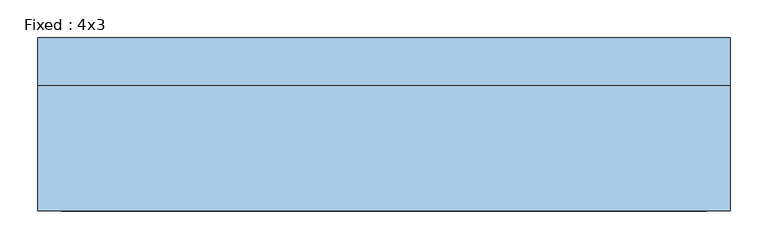
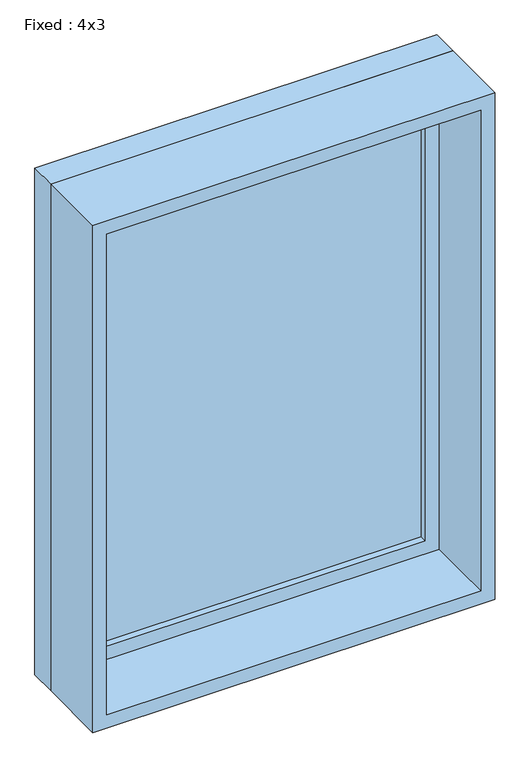
"""IFC4 building model written with IfcOpenShell, lengths in millimetres: window geometry, Fixed : 4x3."""

from ifc_helpers import new_model, si_unit, frame, origin, place, context, project, spatial, polyline, outline, extrude, source, transform, mapped, element, save


def fixed_4x3_c1f32544(model_context):
    return source(origin(), model_context, "Body", "SweptSolid", [
        extrude(outline(polyline([(355.6, 66.675), (-431.8, 66.675), (-431.8, 79.375), (355.6, 79.375), (355.6, 66.675)])), frame((0.0, 0.0, 977.9), z_axis=(0.0, 0.0, 1.0), x_axis=(1.0, 0.0, 0.0)), (0.0, 0.0, 1.0), 1092.2),
        extrude(outline(polyline([(2114.55, -476.25), (933.45, -476.25), (933.45, 400.05), (2114.55, 400.05), (2114.55, -476.25)]), holes=[polyline([(2070.1, -431.8), (2070.1, 355.6), (977.9, 355.6), (977.9, -431.8), (2070.1, -431.8)])]), frame((0.0, 50.8, 0.0), z_axis=(0.0, 1.0, 0.0), x_axis=(0.0, 0.0, 1.0)), (0.0, 0.0, 1.0), 44.45),
        extrude(outline(polyline([(2133.6, -495.3), (914.4, -495.3), (914.4, 419.1), (2133.6, 419.1), (2133.6, -495.3)]), holes=[polyline([(2101.85, -463.55), (2101.85, 387.35), (946.15, 387.35), (946.15, -463.55), (2101.85, -463.55)])]), frame((0.0, -114.3, 0.0), z_axis=(0.0, 1.0, 0.0), x_axis=(0.0, 0.0, 1.0)), (0.0, 0.0, 1.0), 165.1),
        extrude(outline(polyline([(2133.6, 419.1), (2133.6, -495.3), (914.4, -495.3), (914.4, 419.1), (2133.6, 419.1)]), holes=[polyline([(2114.55, 400.05), (933.45, 400.05), (933.45, -476.25), (2114.55, -476.25), (2114.55, 400.05)])]), frame((0.0, 50.8, 0.0), z_axis=(0.0, 1.0, 0.0), x_axis=(0.0, 0.0, 1.0)), (0.0, 0.0, 1.0), 63.5),
    ])


if __name__ == "__main__":
    model = new_model("IFC4")
    model_context = context("Model", 3, world=origin())
    ifc_project = project(units=[si_unit("LENGTHUNIT", "METRE", prefix="MILLI")], contexts=[model_context])
    site = spatial("IfcSite", under=ifc_project)
    building = spatial("IfcBuilding", under=site)
    placement = place(None, origin())
    fixed_4x3_shape = fixed_4x3_c1f32544(model_context)
    element("IfcWindow", 1, ObjectType="Fixed : 4x3", at=placement, inside=building, context=model_context, shape_type="MappedRepresentation", body=[
        mapped(fixed_4x3_shape, transform((0.0, 0.0, 0.0), x_axis=(1.0, 0.0, 0.0), y_axis=(0.0, 1.0, 0.0), z_axis=(0.0, 0.0, 1.0))),
    ])
    save(model, "model.ifc")

# Revit data of these elements
# Type "Fixed : 4x3"
#   Type Mark = "3"
#   Assembly Code = "B2020100"
#   Height = 4' - 0"
#   Default Sill Height = 3' - 0"
#   Width = 3' - 0"
#   Window Inset = 0' - 0 3/4"
#   Glass Pane Material = Glass
#   Sash Material = Sash
#   Wall Closure = (empty or 0)
# Element 1 (IfcWindow, "Fixed : 4x3")
#   Materials on its faces: "Sash", "Glass"
# Materials
#   "Glass": class "Glass", colour RGB 218 227 224, transparency 0.85, Description = "Soda Lime Glass", Cost = 0
#   "Sash": class "Wood", colour RGB 136 99 55, transparency 0
